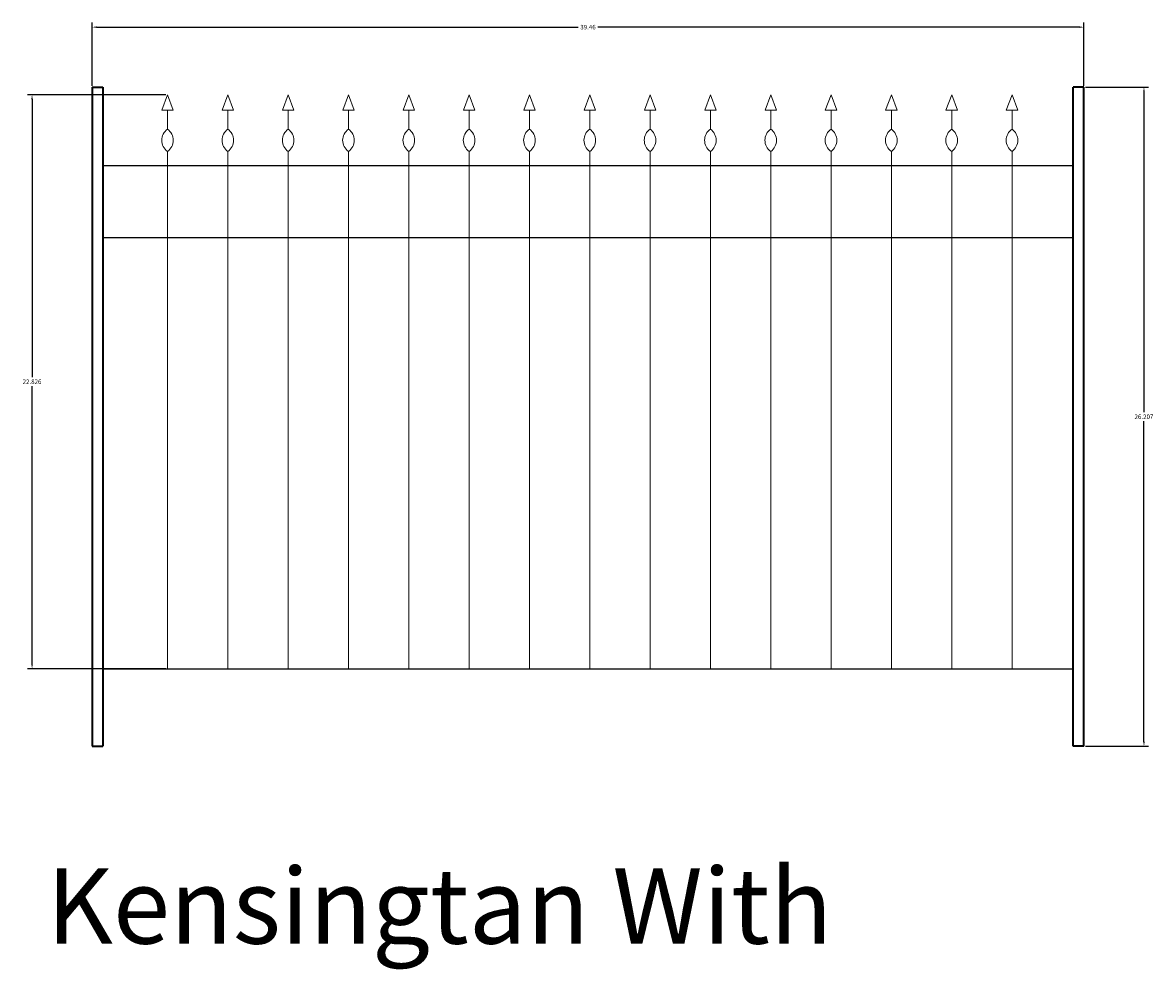
# Model space of a CAD drawing. Units: inches. Extents: x 756 to 915, y 488 to 695.
# Tile 7 of 25: x 814 to 859, y 545 to 583. Entities that reach past the tile are written whole.
import ezdxf

# ---------------------------------------------------------------- set-up
doc = ezdxf.new("R2010")
doc.units = ezdxf.units.IN
doc.header["$MEASUREMENT"] = 0
for name, color, linetype, lineweight in [('L-ANNO-TEXT', 7, 'Continuous', 25), ('L-FENC-PCKT', 7, 'Continuous', 18), ('L-FENC-POST', 7, 'Continuous', 35), ('L-FENC-RAIL', 7, 'Continuous', 25), ('M-DIMS', 2, 'Continuous', 18)]:
    doc.layers.add(name, color=color, linetype=linetype, lineweight=lineweight)
doc.styles.get("Standard").update_dxf_attribs({"font": 'arial.ttf'})
doc.dimstyles.get("Standard").update_dxf_attribs({"dimtxt": 0.18, "dimasz": 0.18, "dimexe": 0.18, "dimexo": 0.0625, "dimgap": 0.09, "dimtad": 0, "dimtih": 1, "dimtoh": 1, "dimdec": 0, "dimzin": 0, "dimdsep": 46, "dimlunit": 3, "dimtxsty": 'Standard', "dimcen": 0.09, "dimadec": 0, "dimazin": 0, "dimtfac": 1, "dimtdec": 0, "dimtofl": 0, "dimtmove": 0, "dimatfit": 3, "dimfxl": 1, "dimtolj": 1, "dimtzin": 0, "dimarcsym": 0})

# ---------------------------------------------------------------- blocks, each defined once
blk = doc.blocks.new('PICKET-MAJESTIC-FLUSH')
for p, q in [((0.231, 22.214), (0.231, 21.456)), ((0.231, 20.573), (0.231, 0))]:
    blk.add_line(p, q)
blk.add_lwpolyline([(0.231, 22.214), (0.004, 22.214), (0.231, 22.826), (0.458, 22.214)], close=True)
blk.add_lwpolyline([(0.231, 20.573, 0.522719), (0.231, 21.456, 0.522719)], format="xyb", close=True)
blk = doc.blocks.new('FENCE-POST-LEFT')
for p, q in [((0, 26.207), (0, 0)), ((0, 26.207), (0.426, 26.207)), ((0.426, 26.207), (0.426, 0)), ((0.426, 26.207), (0.426, 0)), ((0, 0), (0.426, 0))]:
    blk.add_line(p, q)
blk = doc.blocks.new('FENCE-POST-RIGHT')
for p, q in [((0, 26.207), (0, 0)), ((0, 26.207), (0.427, 26.207)), ((0.427, 26.207), (0.427, 0)), ((0, 0), (0.427, 0))]:
    blk.add_line(p, q)
blk = doc.blocks.new('*D69')
at = {"layer": 'Defpoints', "color": 0, "transparency": 16777216}
for p in [(856.101, 582.576), (816.643, 580.186), (856.101, 580.186)]:
    blk.add_point(p, dxfattribs=at)
at = {"layer": 'M-DIMS', "color": 0, "lineweight": -2, "transparency": 16777216}
for p, q in [((816.643, 580.248), (816.643, 582.756)), ((856.101, 580.248), (856.101, 582.756)), ((816.823, 582.576), (835.978, 582.576)), ((855.921, 582.576), (836.765, 582.576))]:
    blk.add_line(p, q, dxfattribs=at)
at = {"layer": 'M-DIMS', "color": 0, "transparency": 16777216}
for points in [[(816.823, 582.606), (816.823, 582.546), (816.643, 582.576)], [(855.921, 582.606), (855.921, 582.546), (856.101, 582.576)]]:
    blk.add_solid(points, dxfattribs=at)
at = {"layer": 'M-DIMS', "color": 0, "transparency": 16777216, "insert": (836.372, 582.576), "char_height": 0.18, "attachment_point": 5}
blk.add_mtext('\\A1;39.46', dxfattribs=at)
blk = doc.blocks.new('*D70')
at = {"layer": 'Defpoints', "color": 0, "transparency": 16777216}
for p in [(856.101, 580.186), (858.491, 580.186), (856.101, 553.979)]:
    blk.add_point(p, dxfattribs=at)
at = {"layer": 'M-DIMS', "color": 0, "lineweight": -2, "transparency": 16777216}
for p, q in [((856.163, 580.186), (858.671, 580.186)), ((858.491, 580.006), (858.491, 567.264)), ((858.491, 554.159), (858.491, 566.9)), ((856.163, 553.979), (858.671, 553.979))]:
    blk.add_line(p, q, dxfattribs=at)
at = {"layer": 'M-DIMS', "color": 0, "transparency": 16777216}
for points in [[(858.461, 580.006), (858.521, 580.006), (858.491, 580.186)], [(858.461, 554.159), (858.521, 554.159), (858.491, 553.979)]]:
    blk.add_solid(points, dxfattribs=at)
at = {"layer": 'M-DIMS', "color": 0, "transparency": 16777216, "insert": (858.491, 567.082), "char_height": 0.18, "attachment_point": 5}
blk.add_mtext('\\A1;26.207', dxfattribs=at)
blk = doc.blocks.new('*D71')
at = {"layer": 'Defpoints', "color": 0, "transparency": 16777216}
for p in [(814.253, 579.887), (819.642, 579.887), (819.642, 557.061)]:
    blk.add_point(p, dxfattribs=at)
at = {"layer": 'M-DIMS', "color": 0, "lineweight": -2, "transparency": 16777216}
for p, q in [((819.579, 579.887), (814.073, 579.887)), ((814.253, 579.707), (814.253, 568.656)), ((814.253, 557.241), (814.253, 568.292)), ((819.579, 557.061), (814.073, 557.061))]:
    blk.add_line(p, q, dxfattribs=at)
at = {"layer": 'M-DIMS', "color": 0, "transparency": 16777216}
for points in [[(814.223, 579.707), (814.283, 579.707), (814.253, 579.887)], [(814.223, 557.241), (814.283, 557.241), (814.253, 557.061)]]:
    blk.add_solid(points, dxfattribs=at)
at = {"layer": 'M-DIMS', "color": 0, "transparency": 16777216, "insert": (814.253, 568.474), "char_height": 0.18, "attachment_point": 5}
blk.add_mtext('\\A1;22.826', dxfattribs=at)

msp = doc.modelspace()

# ---------------------------------------------------------------- linework, layer by layer
at = {"layer": 'L-FENC-RAIL'}
for p, q in [((817.0694, 577.0708), (855.6743, 577.0708)), ((817.0694, 574.2064), (855.6743, 574.2064)), ((817.0694, 557.0606), (855.6743, 557.0606))]:
    msp.add_line(p, q, dxfattribs=at)

# ---------------------------------------------------------------- block references
at = {"layer": 'L-FENC-PCKT'}
for p in [(819.411, 557.061), (821.8109, 557.061), (824.2108, 557.061), (826.6107, 557.061), (829.0106, 557.061), (831.4106, 557.061), (833.8105, 557.061), (836.2104, 557.061), (838.6103, 557.061), (841.0102, 557.061), (843.4101, 557.061), (845.81, 557.061), (848.2099, 557.061), (850.6098, 557.061), (853.0098, 557.061)]:
    msp.add_blockref('PICKET-MAJESTIC-FLUSH', p, dxfattribs=at)
at = {"layer": 'L-FENC-POST'}
msp.add_blockref('FENCE-POST-LEFT', (816.6431, 553.9789), dxfattribs=at)
at = {"layer": 'L-FENC-POST', "rotation": 180}
msp.add_blockref('FENCE-POST-RIGHT', (856.1011, 580.1858), dxfattribs=at)

# ---------------------------------------------------------------- texts
at = {"layer": 'L-ANNO-TEXT'}
msp.add_text('Kensingtan With ', height=3, dxfattribs=at).set_placement((814.829, 546.1271))

# ---------------------------------------------------------------- dimensions: what is measured, and where the dimension line sits
at = {"layer": 'M-DIMS'}
dim = msp.add_linear_dim(base=(856.1009, 582.5758), p1=(816.6428, 580.1858), p2=(856.1009, 580.1858), dimstyle='Standard', override={"dimdec": 2, "dimlfac": 1, "dimrnd": 0, "dimzin": 0, "dimdsep": 46, "dimlunit": 2}, dxfattribs=at)
dim.commit()
dim.dimension.update_dxf_attribs({"geometry": '*D69', "text_midpoint": (836.3719, 582.5758)})
for base, p1, p2, picture, middle in [((858.4909, 580.1858), (856.1009, 553.979), (856.1009, 580.1858), '*D70', (858.4909, 567.0824)), ((814.2528, 579.8867), (819.6419, 557.0606), (819.6419, 579.8867), '*D71', (814.2528, 568.4737))]:
    dim = msp.add_linear_dim(base=base, p1=p1, p2=p2, angle=90, dimstyle='Standard', override={"dimdec": 3, "dimlfac": 1, "dimrnd": 0, "dimzin": 0, "dimdsep": 46, "dimlunit": 2}, dxfattribs=at)
    dim.commit()
    dim.dimension.update_dxf_attribs({"geometry": picture, "text_midpoint": middle})

doc.saveas('drawing.dxf')
